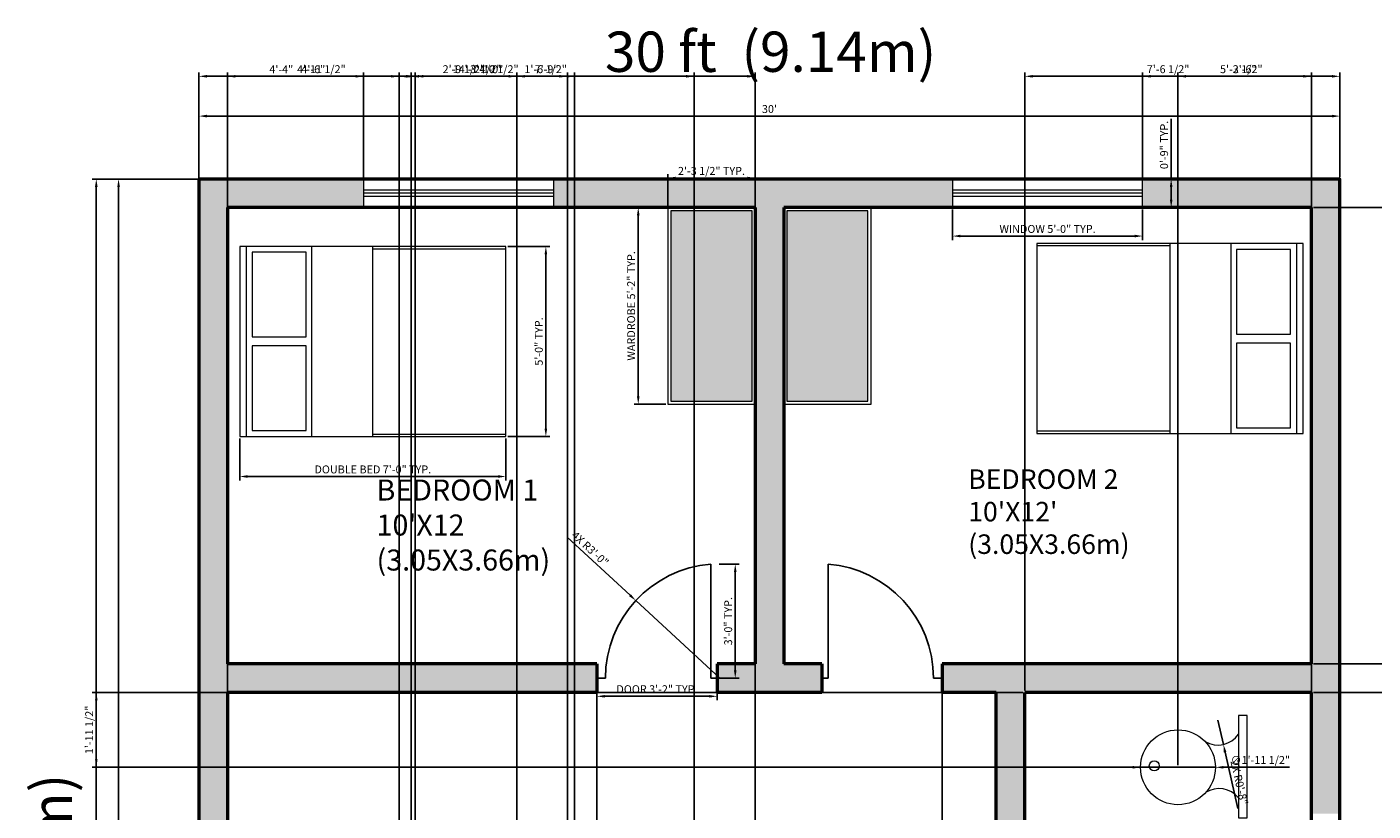
# Model space of a CAD drawing. Units: inches. Extents: x 655 to 1311, y 444 to 1096.
# Tile 3 of 4: x 655 to 1080, y 848 to 1096. Entities that reach past the tile are written whole.
import ezdxf

# ---------------------------------------------------------------- set-up
doc = ezdxf.new("R2010")
doc.units = ezdxf.units.IN
for name, color, linetype, lineweight in [('A-ANNO-DIMS', 7, 'Continuous', 18), ('A-AREA-IDEN', 7, 'Continuous', 18), ('A-COLS-PATT', 7, 'Continuous', 13), ('A-FLOR-FIXT', 8, 'Continuous', 18), ('A-WALL', 7, 'Continuous', 50), ('A-WALL-PATT', 7, 'Continuous', 13)]:
    doc.layers.add(name, color=color, linetype=linetype, lineweight=lineweight)
for name, color, linetype, lineweight, true_color in [('A-DOOR', 251, 'Continuous', 25, 0x636466), ('A-FURN', 251, 'Continuous', 18, 0x636466), ('A-FURN-PATT', 241, 'Continuous', 13, 0xf7abae), ('A-GLAZ', 152, 'Continuous', 18, 0x2776bb)]:
    doc.layers.add(name, color=color, linetype=linetype, lineweight=lineweight, true_color=true_color)
doc.styles.get("Standard").update_dxf_attribs({"font": 'arial.ttf'})
doc.dimstyles.new('ISO-25', dxfattribs={"dimtxt": 2.5, "dimasz": 2.5, "dimexe": 1.25, "dimexo": 0.625, "dimtad": 1, "dimdec": 0, "dimlunit": 3, "dimtxsty": 'Standard', "dimcen": 2.5, "dimadec": 0, "dimazin": 0, "dimtfac": 1, "dimtdec": 0, "dimtmove": 0, "dimatfit": 3, "dimfxl": 1, "dimarcsym": 0})

# ---------------------------------------------------------------- blocks, each defined once
blk = doc.blocks.new('*D1')
at = {"layer": 'A-ANNO-DIMS', "color": 0, "lineweight": -2, "transparency": 16777216}
for p, q in [((709.33, 1048.38), (709.33, 1068.85)), ((711.83, 1067.6), (1066.83, 1067.6)), ((1069.33, 1048.38), (1069.33, 1068.85))]:
    blk.add_line(p, q, dxfattribs=at)
at = {"layer": 'A-ANNO-DIMS', "color": 0, "transparency": 16777216}
for points in [[(711.83, 1068.02), (711.83, 1067.18), (709.33, 1067.6)], [(1066.83, 1068.02), (1066.83, 1067.18), (1069.33, 1067.6)]]:
    blk.add_solid(points, dxfattribs=at)
at = {"layer": 'Defpoints', "color": 0, "transparency": 16777216}
for p in [(1069.33, 1067.6), (709.33, 1047.75), (1069.33, 1047.75)]:
    blk.add_point(p, dxfattribs=at)
at = {"layer": 'A-ANNO-DIMS', "color": 0, "transparency": 16777216, "insert": (889.33, 1069.5), "char_height": 2.5, "attachment_point": 5}
blk.add_mtext("30'", dxfattribs=at)
blk = doc.blocks.new('*D2')
at = {"layer": 'A-ANNO-DIMS', "color": 0, "lineweight": -2, "transparency": 16777216}
for p, q in [((708.71, 1047.75), (682.71, 1047.75)), ((683.96, 570.25), (683.96, 1045.25)), ((708.71, 567.75), (682.71, 567.75))]:
    blk.add_line(p, q, dxfattribs=at)
at = {"layer": 'A-ANNO-DIMS', "color": 0, "transparency": 16777216}
for points in [[(683.55, 1045.25), (684.38, 1045.25), (683.96, 1047.75)], [(683.55, 570.25), (684.38, 570.25), (683.96, 567.75)]]:
    blk.add_solid(points, dxfattribs=at)
at = {"layer": 'Defpoints', "color": 0, "transparency": 16777216}
for p in [(683.96, 1047.75), (709.33, 1047.75), (709.33, 567.75)]:
    blk.add_point(p, dxfattribs=at)
at = {"layer": 'A-ANNO-DIMS', "color": 0, "transparency": 16777216, "insert": (682.06, 807.75), "char_height": 2.5, "attachment_point": 5, "rotation": 90}
blk.add_mtext("40'", dxfattribs=at)
blk = doc.blocks.new('DOOR-SWING-36IN')
for p, q in [((0, 0), (0, 36)), ((-36, 0), (-33.26, 0)), ((0, 0), (2, 0))]:
    blk.add_line(p, q)
blk.add_arc((2.86, 0), 36.11, 94.5377, 180)
blk = doc.blocks.new('WIN-60IN')
for p, q in [((60, 9), (0, 9)), ((0, 9), (0, 0)), ((60, 0), (60, 9)), ((60, 5.5), (0, 5.5)), ((60, 4.5), (0, 4.5)), ((60, 3.5), (0, 3.5)), ((0, 0), (60, 0))]:
    blk.add_line(p, q)
blk = doc.blocks.new('BED-DOUBLE')
for p, q in [((84, 60), (0, 60)), ((0, 60), (0, 0)), ((2, 60), (2, 0)), ((84, 0), (84, 60)), ((42, 59.26), (84, 59.26)), ((0, 0), (84, 0)), ((42, 0.79), (84, 0.79))]:
    blk.add_line(p, q)
for points in [[(42, 0), (42, 60), (22.65, 60), (22.65, 0)], [(20.99, 31.44), (20.99, 58.17), (3.97, 58.17), (3.97, 31.44)], [(20.99, 1.93), (20.99, 28.66), (3.97, 28.66), (3.97, 1.93)]]:
    blk.add_lwpolyline(points, close=True)
blk = doc.blocks.new('WARDROBE-BEDROOM')
for points in [[(27.59, 62.05), (0, 62.05), (0, 0), (27.59, 0)], [(26.59, 61.05), (1, 61.05), (1, 1), (26.59, 1)]]:
    blk.add_lwpolyline(points, close=True)
blk = doc.blocks.new('*D8')
at = {"layer": 'A-ANNO-DIMS', "color": 0, "lineweight": -2, "transparency": 16777216}
for p, q in [((834.83, 889.63), (834.83, 883.3)), ((872.83, 889.63), (872.83, 883.3)), ((837.33, 884.55), (870.33, 884.55))]:
    blk.add_line(p, q, dxfattribs=at)
at = {"layer": 'A-ANNO-DIMS', "color": 0, "transparency": 16777216}
for points in [[(837.33, 884.97), (837.33, 884.14), (834.83, 884.55)], [(870.33, 884.97), (870.33, 884.14), (872.83, 884.55)]]:
    blk.add_solid(points, dxfattribs=at)
at = {"layer": 'Defpoints', "color": 0, "transparency": 16777216}
for p in [(834.83, 890.25), (872.83, 890.25), (872.83, 884.55)]:
    blk.add_point(p, dxfattribs=at)
at = {"layer": 'A-ANNO-DIMS', "color": 0, "transparency": 16777216, "insert": (853.83, 886.47), "char_height": 2.5, "attachment_point": 5}
blk.add_mtext('DOOR 3\'-2" TYP.', dxfattribs=at)
blk = doc.blocks.new('*D9')
at = {"layer": 'A-ANNO-DIMS', "color": 0, "lineweight": -2, "transparency": 16777216}
for p, q in [((873.46, 926.25), (879.78, 926.25)), ((878.53, 892.75), (878.53, 923.75)), ((873.46, 890.25), (879.78, 890.25))]:
    blk.add_line(p, q, dxfattribs=at)
at = {"layer": 'A-ANNO-DIMS', "color": 0, "transparency": 16777216}
for points in [[(878.12, 923.75), (878.95, 923.75), (878.53, 926.25)], [(878.12, 892.75), (878.95, 892.75), (878.53, 890.25)]]:
    blk.add_solid(points, dxfattribs=at)
at = {"layer": 'Defpoints', "color": 0, "transparency": 16777216}
for p in [(872.83, 926.25), (878.53, 926.25), (872.83, 890.25)]:
    blk.add_point(p, dxfattribs=at)
at = {"layer": 'A-ANNO-DIMS', "color": 0, "transparency": 16777216, "insert": (876.63, 908.25), "char_height": 2.5, "attachment_point": 5, "rotation": 90}
blk.add_mtext('3\'-0" TYP.', dxfattribs=at)
blk = doc.blocks.new('*D10')
at = {"layer": 'A-ANNO-DIMS', "color": 0, "lineweight": -2, "transparency": 16777216}
for p, q in [((947.08, 1038.13), (947.08, 1028.5)), ((1007.08, 1038.13), (1007.08, 1028.5)), ((949.58, 1029.75), (1004.58, 1029.75))]:
    blk.add_line(p, q, dxfattribs=at)
at = {"layer": 'A-ANNO-DIMS', "color": 0, "transparency": 16777216}
for points in [[(949.58, 1030.17), (949.58, 1029.34), (947.08, 1029.75)], [(1004.58, 1030.17), (1004.58, 1029.34), (1007.08, 1029.75)]]:
    blk.add_solid(points, dxfattribs=at)
at = {"layer": 'Defpoints', "color": 0, "transparency": 16777216}
for p in [(947.08, 1038.75), (1007.08, 1038.75), (1007.08, 1029.75)]:
    blk.add_point(p, dxfattribs=at)
at = {"layer": 'A-ANNO-DIMS', "color": 0, "transparency": 16777216, "insert": (977.08, 1031.67), "char_height": 2.5, "attachment_point": 5}
blk.add_mtext('WINDOW 5\'-0" TYP.', dxfattribs=at)
blk = doc.blocks.new('*D11')
at = {"layer": 'A-ANNO-DIMS', "color": 0, "lineweight": -2, "transparency": 16777216}
for p, q in [((1016.08, 1047.75), (1016.08, 1066.74)), ((1007.71, 1047.75), (1017.33, 1047.75)), ((1016.08, 1041.25), (1016.08, 1045.25)), ((1007.71, 1038.75), (1017.33, 1038.75))]:
    blk.add_line(p, q, dxfattribs=at)
at = {"layer": 'A-ANNO-DIMS', "color": 0, "transparency": 16777216}
for points in [[(1015.67, 1045.25), (1016.5, 1045.25), (1016.08, 1047.75)], [(1015.67, 1041.25), (1016.5, 1041.25), (1016.08, 1038.75)]]:
    blk.add_solid(points, dxfattribs=at)
at = {"layer": 'Defpoints', "color": 0, "transparency": 16777216}
for p in [(1007.08, 1047.75), (1016.08, 1047.75), (1007.08, 1038.75)]:
    blk.add_point(p, dxfattribs=at)
at = {"layer": 'A-ANNO-DIMS', "color": 0, "transparency": 16777216, "insert": (1014.18, 1058.5), "char_height": 2.5, "attachment_point": 5, "rotation": 90}
blk.add_mtext('0\'-9" TYP.', dxfattribs=at)
blk = doc.blocks.new('*D12')
at = {"layer": 'A-ANNO-DIMS', "color": 0, "lineweight": -2, "transparency": 16777216}
for p, q in [((722.18, 965.87), (722.18, 952.64)), ((806.18, 965.87), (806.18, 952.64)), ((724.68, 953.89), (803.68, 953.89))]:
    blk.add_line(p, q, dxfattribs=at)
at = {"layer": 'A-ANNO-DIMS', "color": 0, "transparency": 16777216}
for points in [[(724.68, 954.31), (724.68, 953.48), (722.18, 953.89)], [(803.68, 954.31), (803.68, 953.48), (806.18, 953.89)]]:
    blk.add_solid(points, dxfattribs=at)
at = {"layer": 'Defpoints', "color": 0, "transparency": 16777216}
for p in [(722.18, 966.49), (806.18, 966.49), (806.18, 953.89)]:
    blk.add_point(p, dxfattribs=at)
at = {"layer": 'A-ANNO-DIMS', "color": 0, "transparency": 16777216, "insert": (764.18, 955.81), "char_height": 2.5, "attachment_point": 5}
blk.add_mtext('DOUBLE BED 7\'-0" TYP.', dxfattribs=at)
blk = doc.blocks.new('*D13')
at = {"layer": 'A-ANNO-DIMS', "color": 0, "lineweight": -2, "transparency": 16777216}
for p, q in [((806.8, 1026.49), (820.03, 1026.49)), ((818.78, 968.99), (818.78, 1023.99)), ((806.8, 966.49), (820.03, 966.49))]:
    blk.add_line(p, q, dxfattribs=at)
at = {"layer": 'A-ANNO-DIMS', "color": 0, "transparency": 16777216}
for points in [[(818.36, 1023.99), (819.19, 1023.99), (818.78, 1026.49)], [(818.36, 968.99), (819.19, 968.99), (818.78, 966.49)]]:
    blk.add_solid(points, dxfattribs=at)
at = {"layer": 'Defpoints', "color": 0, "transparency": 16777216}
for p in [(806.18, 1026.49), (818.78, 1026.49), (806.18, 966.49)]:
    blk.add_point(p, dxfattribs=at)
at = {"layer": 'A-ANNO-DIMS', "color": 0, "transparency": 16777216, "insert": (816.88, 996.49), "char_height": 2.5, "attachment_point": 5, "rotation": 90}
blk.add_mtext('5\'-0" TYP.', dxfattribs=at)
blk = doc.blocks.new('*D14')
at = {"layer": 'A-ANNO-DIMS', "color": 0, "lineweight": -2, "transparency": 16777216}
for p, q in [((856.62, 1038.75), (846.68, 1038.75)), ((847.93, 979.2), (847.93, 1036.25)), ((856.62, 976.7), (846.68, 976.7))]:
    blk.add_line(p, q, dxfattribs=at)
at = {"layer": 'A-ANNO-DIMS', "color": 0, "transparency": 16777216}
for points in [[(847.52, 1036.25), (848.35, 1036.25), (847.93, 1038.75)], [(847.52, 979.2), (848.35, 979.2), (847.93, 976.7)]]:
    blk.add_solid(points, dxfattribs=at)
at = {"layer": 'Defpoints', "color": 0, "transparency": 16777216}
for p in [(847.93, 1038.75), (857.24, 1038.75), (857.24, 976.7)]:
    blk.add_point(p, dxfattribs=at)
at = {"layer": 'A-ANNO-DIMS', "color": 0, "transparency": 16777216, "insert": (846.01, 1007.73), "char_height": 2.5, "attachment_point": 5, "rotation": 90}
blk.add_mtext('WARDROBE 5\'-2" TYP.', dxfattribs=at)
blk = doc.blocks.new('*D15')
at = {"layer": 'A-ANNO-DIMS', "color": 0, "lineweight": -2, "transparency": 16777216}
for p, q in [((857.24, 1039.38), (857.24, 1049.31)), ((884.83, 1039.38), (884.83, 1049.31)), ((859.74, 1048.06), (882.33, 1048.06))]:
    blk.add_line(p, q, dxfattribs=at)
at = {"layer": 'A-ANNO-DIMS', "color": 0, "transparency": 16777216}
for points in [[(859.74, 1048.48), (859.74, 1047.64), (857.24, 1048.06)], [(882.33, 1048.48), (882.33, 1047.64), (884.83, 1048.06)]]:
    blk.add_solid(points, dxfattribs=at)
at = {"layer": 'Defpoints', "color": 0, "transparency": 16777216}
for p in [(884.83, 1048.06), (857.24, 1038.75), (884.83, 1038.75)]:
    blk.add_point(p, dxfattribs=at)
at = {"layer": 'A-ANNO-DIMS', "color": 0, "transparency": 16777216, "insert": (871.04, 1049.98), "char_height": 2.5, "attachment_point": 5}
blk.add_mtext('2\'-3 1/2" TYP.', dxfattribs=at)
blk = doc.blocks.new('*D18')
at = {"layer": 'A-ANNO-DIMS', "color": 0, "lineweight": -2, "transparency": 16777216}
for p, q in [((718.33, 1039.38), (718.33, 1081.4)), ((720.83, 1080.15), (882.33, 1080.15)), ((884.83, 1039.38), (884.83, 1081.4))]:
    blk.add_line(p, q, dxfattribs=at)
at = {"layer": 'A-ANNO-DIMS', "color": 0, "transparency": 16777216}
for points in [[(720.83, 1080.57), (720.83, 1079.74), (718.33, 1080.15)], [(882.33, 1080.57), (882.33, 1079.74), (884.83, 1080.15)]]:
    blk.add_solid(points, dxfattribs=at)
at = {"layer": 'Defpoints', "color": 0, "transparency": 16777216}
for p in [(884.83, 1080.15), (718.33, 1038.75), (884.83, 1038.75)]:
    blk.add_point(p, dxfattribs=at)
at = {"layer": 'A-ANNO-DIMS', "color": 0, "transparency": 16777216, "insert": (801.58, 1082.07), "char_height": 2.5, "attachment_point": 5}
blk.add_mtext('13\'-10 1/2"', dxfattribs=at)
blk = doc.blocks.new('*D19')
at = {"layer": 'A-ANNO-DIMS', "color": 0, "lineweight": -2, "transparency": 16777216}
for p, q in [((709.33, 1048.38), (709.33, 1081.4)), ((711.83, 1080.15), (758.77, 1080.15)), ((761.27, 1048.38), (761.27, 1081.4))]:
    blk.add_line(p, q, dxfattribs=at)
at = {"layer": 'A-ANNO-DIMS', "color": 0, "transparency": 16777216}
for points in [[(711.83, 1080.57), (711.83, 1079.74), (709.33, 1080.15)], [(758.77, 1080.57), (758.77, 1079.74), (761.27, 1080.15)]]:
    blk.add_solid(points, dxfattribs=at)
at = {"layer": 'Defpoints', "color": 0, "transparency": 16777216}
for p in [(761.27, 1080.15), (709.33, 1047.75), (761.27, 1047.75)]:
    blk.add_point(p, dxfattribs=at)
at = {"layer": 'A-ANNO-DIMS', "color": 0, "transparency": 16777216, "insert": (735.3, 1082.03), "char_height": 2.5, "attachment_point": 5}
blk.add_mtext('4\'-4"', dxfattribs=at)
blk = doc.blocks.new('*D20')
at = {"layer": 'A-ANNO-DIMS', "color": 0, "lineweight": -2, "transparency": 16777216}
for p, q in [((1007.08, 1048.38), (1007.08, 1081.4)), ((1009.58, 1080.15), (1066.83, 1080.15)), ((1069.33, 1048.38), (1069.33, 1081.4))]:
    blk.add_line(p, q, dxfattribs=at)
at = {"layer": 'A-ANNO-DIMS', "color": 0, "transparency": 16777216}
for points in [[(1009.58, 1080.57), (1009.58, 1079.74), (1007.08, 1080.15)], [(1066.83, 1080.57), (1066.83, 1079.74), (1069.33, 1080.15)]]:
    blk.add_solid(points, dxfattribs=at)
at = {"layer": 'Defpoints', "color": 0, "transparency": 16777216}
for p in [(1069.33, 1080.15), (1007.08, 1047.75), (1069.33, 1047.75)]:
    blk.add_point(p, dxfattribs=at)
at = {"layer": 'A-ANNO-DIMS', "color": 0, "transparency": 16777216, "insert": (1038.21, 1082.07), "char_height": 2.5, "attachment_point": 5}
blk.add_mtext('5\'-2 1/2"', dxfattribs=at)
blk = doc.blocks.new('*D21')
at = {"layer": 'A-ANNO-DIMS', "color": 0, "lineweight": -2, "transparency": 16777216}
for p, q in [((718.33, 894.13), (718.33, 444.55)), ((834.83, 894.13), (834.83, 444.55)), ((720.83, 445.8), (832.33, 445.8))]:
    blk.add_line(p, q, dxfattribs=at)
at = {"layer": 'A-ANNO-DIMS', "color": 0, "transparency": 16777216}
for points in [[(720.83, 446.22), (720.83, 445.38), (718.33, 445.8)], [(832.33, 446.22), (832.33, 445.38), (834.83, 445.8)]]:
    blk.add_solid(points, dxfattribs=at)
at = {"layer": 'Defpoints', "color": 0, "transparency": 16777216}
for p in [(718.33, 894.75), (834.83, 894.75), (834.83, 445.8)]:
    blk.add_point(p, dxfattribs=at)
at = {"layer": 'A-ANNO-DIMS', "color": 0, "transparency": 16777216, "insert": (776.58, 447.72), "char_height": 2.5, "attachment_point": 5}
blk.add_mtext('9\'-8 1/2"', dxfattribs=at)
blk = doc.blocks.new('*D22')
at = {"layer": 'A-ANNO-DIMS', "color": 0, "lineweight": -2, "transparency": 16777216}
for p, q in [((943.83, 894.13), (943.83, 444.55)), ((1060.33, 894.13), (1060.33, 444.55)), ((946.33, 445.8), (1057.83, 445.8))]:
    blk.add_line(p, q, dxfattribs=at)
at = {"layer": 'A-ANNO-DIMS', "color": 0, "transparency": 16777216}
for points in [[(946.33, 446.22), (946.33, 445.38), (943.83, 445.8)], [(1057.83, 446.22), (1057.83, 445.38), (1060.33, 445.8)]]:
    blk.add_solid(points, dxfattribs=at)
at = {"layer": 'Defpoints', "color": 0, "transparency": 16777216}
for p in [(943.83, 894.75), (1060.33, 894.75), (1060.33, 445.8)]:
    blk.add_point(p, dxfattribs=at)
at = {"layer": 'A-ANNO-DIMS', "color": 0, "transparency": 16777216, "insert": (1002.08, 447.72), "char_height": 2.5, "attachment_point": 5}
blk.add_mtext('9\'-8 1/2"', dxfattribs=at)
blk = doc.blocks.new('*D23')
at = {"layer": 'A-ANNO-DIMS', "color": 0, "lineweight": -2, "transparency": 16777216}
for p, q in [((1060.96, 1038.75), (1102.98, 1038.75)), ((1101.73, 897.25), (1101.73, 1036.25)), ((1060.96, 894.75), (1102.98, 894.75))]:
    blk.add_line(p, q, dxfattribs=at)
at = {"layer": 'A-ANNO-DIMS', "color": 0, "transparency": 16777216}
for points in [[(1101.32, 1036.25), (1102.15, 1036.25), (1101.73, 1038.75)], [(1101.32, 897.25), (1102.15, 897.25), (1101.73, 894.75)]]:
    blk.add_solid(points, dxfattribs=at)
at = {"layer": 'Defpoints', "color": 0, "transparency": 16777216}
for p in [(1060.33, 1038.75), (1101.73, 1038.75), (1060.33, 894.75)]:
    blk.add_point(p, dxfattribs=at)
at = {"layer": 'A-ANNO-DIMS', "color": 0, "transparency": 16777216, "insert": (1099.83, 966.75), "char_height": 2.5, "attachment_point": 5, "rotation": 90}
blk.add_mtext('12\'-0"', dxfattribs=at)
blk = doc.blocks.new('*D24')
at = {"layer": 'A-ANNO-DIMS', "color": 0, "lineweight": -2, "transparency": 16777216}
for p, q in [((969.89, 886.38), (969.89, 1081.4)), ((972.39, 1080.15), (1057.83, 1080.15)), ((1060.33, 886.38), (1060.33, 1081.4))]:
    blk.add_line(p, q, dxfattribs=at)
at = {"layer": 'A-ANNO-DIMS', "color": 0, "transparency": 16777216}
for points in [[(972.39, 1080.57), (972.39, 1079.74), (969.89, 1080.15)], [(1057.83, 1080.57), (1057.83, 1079.74), (1060.33, 1080.15)]]:
    blk.add_solid(points, dxfattribs=at)
at = {"layer": 'Defpoints', "color": 0, "transparency": 16777216}
for p in [(1060.33, 1080.15), (969.89, 885.75), (1060.33, 885.75)]:
    blk.add_point(p, dxfattribs=at)
at = {"layer": 'A-ANNO-DIMS', "color": 0, "transparency": 16777216, "insert": (1015.11, 1082.07), "char_height": 2.5, "attachment_point": 5}
blk.add_mtext('7\'-6 1/2"', dxfattribs=at)
blk = doc.blocks.new('*D25')
at = {"layer": 'A-ANNO-DIMS', "color": 0, "lineweight": -2, "transparency": 16777216}
for p, q in [((1060.96, 885.75), (1102.98, 885.75)), ((1101.73, 765.73), (1101.73, 883.25)), ((1060.96, 763.23), (1102.98, 763.23))]:
    blk.add_line(p, q, dxfattribs=at)
at = {"layer": 'A-ANNO-DIMS', "color": 0, "transparency": 16777216}
for points in [[(1101.32, 883.25), (1102.15, 883.25), (1101.73, 885.75)], [(1101.32, 765.73), (1102.15, 765.73), (1101.73, 763.23)]]:
    blk.add_solid(points, dxfattribs=at)
at = {"layer": 'Defpoints', "color": 0, "transparency": 16777216}
for p in [(1060.33, 885.75), (1101.73, 885.75), (1060.33, 763.23)]:
    blk.add_point(p, dxfattribs=at)
at = {"layer": 'A-ANNO-DIMS', "color": 0, "transparency": 16777216, "insert": (1099.81, 824.49), "char_height": 2.5, "attachment_point": 5, "rotation": 90}
blk.add_mtext('10\'-2 1/2"', dxfattribs=at)
blk = doc.blocks.new('*D34')
at = {"layer": 'A-ANNO-DIMS', "color": 0, "lineweight": -2, "transparency": 16777216}
for p, q in [((1018.22, 862.78), (1018.22, 1081.4)), ((1020.72, 1080.15), (1057.83, 1080.15)), ((1060.33, 886.38), (1060.33, 1081.4))]:
    blk.add_line(p, q, dxfattribs=at)
at = {"layer": 'A-ANNO-DIMS', "color": 0, "transparency": 16777216}
for points in [[(1020.72, 1080.57), (1020.72, 1079.74), (1018.22, 1080.15)], [(1057.83, 1080.57), (1057.83, 1079.74), (1060.33, 1080.15)]]:
    blk.add_solid(points, dxfattribs=at)
at = {"layer": 'Defpoints', "color": 0, "transparency": 16777216}
for p in [(1060.33, 1080.15), (1060.33, 885.75), (1018.22, 862.16)]:
    blk.add_point(p, dxfattribs=at)
at = {"layer": 'A-ANNO-DIMS', "color": 0, "transparency": 16777216, "insert": (1039.27, 1082.06), "char_height": 2.5, "attachment_point": 5}
blk.add_mtext('3\'-6"', dxfattribs=at)
blk = doc.blocks.new('*D35')
at = {"layer": 'A-ANNO-DIMS', "color": 0, "lineweight": -2, "transparency": 16777216}
for p, q in [((969.27, 885.75), (675.68, 885.75)), ((676.93, 864.66), (676.93, 883.25)), ((1017.59, 862.16), (675.68, 862.16))]:
    blk.add_line(p, q, dxfattribs=at)
at = {"layer": 'A-ANNO-DIMS', "color": 0, "transparency": 16777216}
for points in [[(676.52, 883.25), (677.35, 883.25), (676.93, 885.75)], [(676.52, 864.66), (677.35, 864.66), (676.93, 862.16)]]:
    blk.add_solid(points, dxfattribs=at)
at = {"layer": 'Defpoints', "color": 0, "transparency": 16777216}
for p in [(676.93, 885.75), (969.89, 885.75), (1018.22, 862.16)]:
    blk.add_point(p, dxfattribs=at)
at = {"layer": 'A-ANNO-DIMS', "color": 0, "transparency": 16777216, "insert": (675.01, 873.96), "char_height": 2.5, "attachment_point": 5, "rotation": 90}
blk.add_mtext('1\'-11 1/2"', dxfattribs=at)
blk = doc.blocks.new('*D48')
at = {"layer": 'A-ANNO-DIMS', "color": 0, "lineweight": -2, "transparency": 16777216}
for p, q in [((709.33, 568.38), (709.33, 1081.4)), ((711.83, 1080.15), (882.33, 1080.15)), ((884.83, 568.38), (884.83, 1081.4))]:
    blk.add_line(p, q, dxfattribs=at)
at = {"layer": 'A-ANNO-DIMS', "color": 0, "transparency": 16777216}
for points in [[(711.83, 1080.57), (711.83, 1079.74), (709.33, 1080.15)], [(882.33, 1080.57), (882.33, 1079.74), (884.83, 1080.15)]]:
    blk.add_solid(points, dxfattribs=at)
at = {"layer": 'Defpoints', "color": 0, "transparency": 16777216}
for p in [(884.83, 1080.15), (709.33, 567.75), (884.83, 567.75)]:
    blk.add_point(p, dxfattribs=at)
at = {"layer": 'A-ANNO-DIMS', "color": 0, "transparency": 16777216, "insert": (797.08, 1082.07), "char_height": 2.5, "attachment_point": 5}
blk.add_mtext('14\'-7 1/2"', dxfattribs=at)
blk = doc.blocks.new('*D51')
at = {"layer": 'A-ANNO-DIMS', "color": 0, "lineweight": -2, "transparency": 16777216}
for p, q in [((718.33, 559.38), (718.33, 1081.4)), ((720.83, 1080.15), (775.08, 1080.15)), ((777.58, 559.38), (777.58, 1081.4))]:
    blk.add_line(p, q, dxfattribs=at)
at = {"layer": 'A-ANNO-DIMS', "color": 0, "transparency": 16777216}
for points in [[(720.83, 1080.57), (720.83, 1079.74), (718.33, 1080.15)], [(775.08, 1080.57), (775.08, 1079.74), (777.58, 1080.15)]]:
    blk.add_solid(points, dxfattribs=at)
at = {"layer": 'Defpoints', "color": 0, "transparency": 16777216}
for p in [(777.58, 1080.15), (718.33, 558.75), (777.58, 558.75)]:
    blk.add_point(p, dxfattribs=at)
at = {"layer": 'A-ANNO-DIMS', "color": 0, "transparency": 16777216, "insert": (747.96, 1082.07), "char_height": 2.5, "attachment_point": 5}
blk.add_mtext('4\'-11 1/2"', dxfattribs=at)
blk = doc.blocks.new('*D53')
at = {"layer": 'A-ANNO-DIMS', "color": 0, "lineweight": -2, "transparency": 16777216}
for p, q in [((777.58, 527.53), (777.58, 1081.4)), ((780.08, 1080.15), (823.08, 1080.15)), ((825.58, 527.53), (825.58, 1081.4))]:
    blk.add_line(p, q, dxfattribs=at)
at = {"layer": 'A-ANNO-DIMS', "color": 0, "transparency": 16777216}
for points in [[(780.08, 1080.57), (780.08, 1079.74), (777.58, 1080.15)], [(823.08, 1080.57), (823.08, 1079.74), (825.58, 1080.15)]]:
    blk.add_solid(points, dxfattribs=at)
at = {"layer": 'Defpoints', "color": 0, "transparency": 16777216}
for p in [(825.58, 1080.15), (777.58, 526.9), (825.58, 526.9)]:
    blk.add_point(p, dxfattribs=at)
at = {"layer": 'A-ANNO-DIMS', "color": 0, "transparency": 16777216, "insert": (801.58, 1082.05), "char_height": 2.5, "attachment_point": 5}
blk.add_mtext('4\'-0"', dxfattribs=at)
blk = doc.blocks.new('*D54')
at = {"layer": 'A-ANNO-DIMS', "color": 0, "lineweight": -2, "transparency": 16777216}
for p, q in [((708.71, 1047.75), (675.68, 1047.75)), ((676.93, 480.7), (676.93, 1045.25)), ((708.71, 478.2), (675.68, 478.2))]:
    blk.add_line(p, q, dxfattribs=at)
at = {"layer": 'A-ANNO-DIMS', "color": 0, "transparency": 16777216}
for points in [[(676.52, 1045.25), (677.35, 1045.25), (676.93, 1047.75)], [(676.52, 480.7), (677.35, 480.7), (676.93, 478.2)]]:
    blk.add_solid(points, dxfattribs=at)
at = {"layer": 'Defpoints', "color": 0, "transparency": 16777216}
for p in [(676.93, 1047.75), (709.33, 1047.75), (709.33, 478.2)]:
    blk.add_point(p, dxfattribs=at)
at = {"layer": 'A-ANNO-DIMS', "color": 0, "transparency": 16777216, "insert": (675.01, 762.98), "char_height": 2.5, "attachment_point": 5, "rotation": 90}
blk.add_mtext('47\'-5 1/2"', dxfattribs=at)
blk = doc.blocks.new('*D55')
at = {"layer": 'A-ANNO-DIMS', "color": 0, "lineweight": -2, "transparency": 16777216}
for p, q in [((772.49, 690.25), (772.49, 1081.4)), ((774.99, 1080.15), (863.04, 1080.15)), ((865.54, 690.25), (865.54, 1081.4))]:
    blk.add_line(p, q, dxfattribs=at)
at = {"layer": 'A-ANNO-DIMS', "color": 0, "transparency": 16777216}
for points in [[(774.99, 1080.57), (774.99, 1079.74), (772.49, 1080.15)], [(863.04, 1080.57), (863.04, 1079.74), (865.54, 1080.15)]]:
    blk.add_solid(points, dxfattribs=at)
at = {"layer": 'Defpoints', "color": 0, "transparency": 16777216}
for p in [(865.54, 1080.15), (772.49, 689.62), (865.54, 689.62)]:
    blk.add_point(p, dxfattribs=at)
at = {"layer": 'A-ANNO-DIMS', "color": 0, "transparency": 16777216, "insert": (819.01, 1082.05), "char_height": 2.5, "attachment_point": 5}
blk.add_mtext('7\'-9"', dxfattribs=at)
blk = doc.blocks.new('*D57')
at = {"layer": 'A-ANNO-DIMS', "color": 0, "lineweight": -2, "transparency": 16777216}
for p, q in [((776.25, 816.16), (776.25, 1081.4)), ((778.75, 1080.15), (807.08, 1080.15)), ((809.58, 816.16), (809.58, 1081.4))]:
    blk.add_line(p, q, dxfattribs=at)
at = {"layer": 'A-ANNO-DIMS', "color": 0, "transparency": 16777216}
for points in [[(778.75, 1080.57), (778.75, 1079.74), (776.25, 1080.15)], [(807.08, 1080.57), (807.08, 1079.74), (809.58, 1080.15)]]:
    blk.add_solid(points, dxfattribs=at)
at = {"layer": 'Defpoints', "color": 0, "transparency": 16777216}
for p in [(809.58, 1080.15), (776.25, 815.54), (809.58, 815.54)]:
    blk.add_point(p, dxfattribs=at)
at = {"layer": 'A-ANNO-DIMS', "color": 0, "transparency": 16777216, "insert": (792.91, 1082.07), "char_height": 2.5, "attachment_point": 5}
blk.add_mtext('2\'-9 1/2"', dxfattribs=at)
blk = doc.blocks.new('*D59')
at = {"layer": 'A-ANNO-DIMS', "color": 0, "lineweight": -2, "transparency": 16777216}
for p, q in [((718.33, 658.38), (718.33, 1081.4)), ((720.83, 1080.15), (769.99, 1080.15)), ((772.49, 690.25), (772.49, 1081.4))]:
    blk.add_line(p, q, dxfattribs=at)
at = {"layer": 'A-ANNO-DIMS', "color": 0, "transparency": 16777216}
for points in [[(720.83, 1080.57), (720.83, 1079.74), (718.33, 1080.15)], [(769.99, 1080.57), (769.99, 1079.74), (772.49, 1080.15)]]:
    blk.add_solid(points, dxfattribs=at)
at = {"layer": 'Defpoints', "color": 0, "transparency": 16777216}
for p in [(772.49, 1080.15), (772.49, 689.62), (718.33, 657.75)]:
    blk.add_point(p, dxfattribs=at)
at = {"layer": 'A-ANNO-DIMS', "color": 0, "transparency": 16777216, "insert": (745.41, 1082.05), "char_height": 2.5, "attachment_point": 5}
blk.add_mtext('4\'-6"', dxfattribs=at)
blk = doc.blocks.new('*D61')
at = {"layer": 'A-ANNO-DIMS', "color": 0, "lineweight": -2, "transparency": 16777216}
for p, q in [((809.58, 816.16), (809.58, 1081.4)), ((812.08, 1080.15), (825.34, 1080.15)), ((827.84, 831.58), (827.84, 1081.4))]:
    blk.add_line(p, q, dxfattribs=at)
at = {"layer": 'A-ANNO-DIMS', "color": 0, "transparency": 16777216}
for points in [[(812.08, 1080.57), (812.08, 1079.74), (809.58, 1080.15)], [(825.34, 1080.57), (825.34, 1079.74), (827.84, 1080.15)]]:
    blk.add_solid(points, dxfattribs=at)
at = {"layer": 'Defpoints', "color": 0, "transparency": 16777216}
for p in [(827.84, 1080.15), (827.84, 830.95), (809.58, 815.54)]:
    blk.add_point(p, dxfattribs=at)
at = {"layer": 'A-ANNO-DIMS', "color": 0, "transparency": 16777216, "insert": (818.71, 1082.07), "char_height": 2.5, "attachment_point": 5}
blk.add_mtext('1\'-6 1/2"', dxfattribs=at)
blk = doc.blocks.new('*D63')
at = {"layer": 'A-ANNO-DIMS', "color": 0, "lineweight": -2, "transparency": 16777216}
for p, q in [((825.46, 934.81), (845.33, 916.45)), ((873.69, 890.25), (847.16, 914.76))]:
    blk.add_line(p, q, dxfattribs=at)
at = {"layer": 'A-ANNO-DIMS', "color": 0, "transparency": 16777216}
blk.add_solid([(845.61, 916.76), (845.04, 916.15), (847.16, 914.76)], dxfattribs=at)
at = {"layer": 'Defpoints', "color": 0, "transparency": 16777216}
for p in [(847.16, 914.76), (873.69, 890.25)]:
    blk.add_point(p, dxfattribs=at)
at = {"layer": 'A-ANNO-DIMS', "color": 0, "transparency": 16777216, "insert": (832.54, 930.86), "char_height": 2.5, "attachment_point": 5, "rotation": 317.2687}
blk.add_mtext('4X R3\'-0"', dxfattribs=at)
blk = doc.blocks.new('*D65')
at = {"layer": 'A-ANNO-DIMS', "color": 0, "lineweight": -2, "transparency": 16777216}
for p, q in [((1003.9, 862.16), (1001.4, 862.16)), ((1006.4, 862.16), (1030.04, 862.16)), ((1053.42, 862.16), (1032.54, 862.16))]:
    blk.add_line(p, q, dxfattribs=at)
at = {"layer": 'A-ANNO-DIMS', "color": 0, "transparency": 16777216}
for points in [[(1003.9, 862.58), (1003.9, 861.74), (1006.4, 862.16)], [(1032.54, 862.57), (1032.54, 861.74), (1030.04, 862.16)]]:
    blk.add_solid(points, dxfattribs=at)
at = {"layer": 'Defpoints', "color": 0, "transparency": 16777216}
for p in [(1006.4, 862.16), (1030.04, 862.16)]:
    blk.add_point(p, dxfattribs=at)
at = {"layer": 'A-ANNO-DIMS', "color": 0, "transparency": 16777216, "insert": (1044.23, 864.13), "char_height": 2.5, "attachment_point": 5, "rotation": 359.9987}
blk.add_mtext('∅1\'-11 1/2"', dxfattribs=at)
blk = doc.blocks.new('*D66')
at = {"layer": 'A-ANNO-DIMS', "color": 0, "lineweight": -2, "transparency": 16777216}
for p, q in [((1030.8, 877.06), (1032.55, 869.37)), ((1037.16, 849.19), (1033.11, 866.93))]:
    blk.add_line(p, q, dxfattribs=at)
at = {"layer": 'A-ANNO-DIMS', "color": 0, "transparency": 16777216}
blk.add_solid([(1033.52, 867.03), (1032.7, 866.84), (1032.55, 869.37)], dxfattribs=at)
at = {"layer": 'Defpoints', "color": 0, "transparency": 16777216}
for p in [(1030.8, 877.06), (1032.55, 869.37)]:
    blk.add_point(p, dxfattribs=at)
at = {"layer": 'A-ANNO-DIMS', "color": 0, "transparency": 16777216, "insert": (1037.26, 857.26), "char_height": 2.5, "attachment_point": 5, "rotation": 282.8435}
blk.add_mtext('2X R0\'-8"', dxfattribs=at)

msp = doc.modelspace()

# ---------------------------------------------------------------- hatches: boundary and pattern name
at = {"layer": 'A-COLS-PATT'}
h = msp.add_hatch(color=256, dxfattribs=at)
h.dxf.hatch_style = 1
h.paths.add_polyline_path([(718.33, 558.75), (718.33, 567.75), (709.33, 567.75), (709.33, 558.75)])
h.paths.add_polyline_path([(893.83, 567.75), (884.83, 567.75), (884.83, 558.75), (893.83, 558.75)])
h.paths.add_polyline_path([(875.1, 756.19), (944.53, 756.19), (944.53, 796.18), (875.1, 796.18)], flags=9)
h.paths.add_polyline_path([(997.04, 810.04), (1045.86, 810.04), (1045.86, 839.51), (997.04, 839.51)], flags=9)
h.paths.add_polyline_path([(949.57, 925.87), (1005.17, 925.87), (1005.17, 959.21), (949.57, 959.21)], flags=9)
h.paths.add_polyline_path([(762.7, 920.37), (822.54, 920.37), (822.54, 956.25), (762.7, 956.25)], flags=9)
at = {"layer": 'A-FURN-PATT'}
h = msp.add_hatch(color=256, dxfattribs=at)
h.dxf.hatch_style = 1
h.paths.add_polyline_path([(883.83, 1037.75), (858.24, 1037.75), (858.24, 977.7), (883.83, 977.7)])
h.paths.add_polyline_path([(920.42, 1037.75), (894.83, 1037.75), (894.83, 977.7), (920.42, 977.7)])
at = {"layer": 'A-WALL-PATT'}
h = msp.add_hatch(color=256, dxfattribs=at)
h.dxf.hatch_style = 1
h.paths.add_polyline_path([(969.89, 885.75), (1060.33, 885.75), (1060.33, 847.5), (1069.33, 847.5), (1069.33, 1047.75), (1007.08, 1047.75), (1007.08, 1038.75), (1060.33, 1038.75), (1060.33, 894.75), (943.83, 894.75), (943.83, 885.75), (960.89, 885.75), (960.89, 822.23), (969.89, 822.23)])
h.paths.add_polyline_path([(969.89, 780.75), (969.89, 790.23), (960.89, 790.23), (960.89, 733.85), (893.83, 733.85), (893.83, 695.8), (902.83, 695.71), (902.83, 724.85), (969.89, 724.85), (969.89, 754.19), (1060.33, 754.19), (1060.33, 699.99), (1069.33, 699.99), (1069.33, 823.5), (1060.33, 823.5), (1060.33, 763.19), (969.89, 763.19)])
h.paths.add_polyline_path([(947.08, 1047.75), (821.27, 1047.75), (821.27, 1038.75), (884.83, 1038.75), (884.83, 976.7), (884.83, 894.75), (872.83, 894.75), (872.83, 885.75), (905.83, 885.75), (905.83, 894.75), (893.83, 894.75), (893.83, 1038.75), (921.42, 1038.75), (947.08, 1038.75)])
h.paths.add_polyline_path([(761.27, 1047.75), (709.33, 1047.75), (709.33, 648.75), (736.08, 648.75), (736.08, 657.75), (718.33, 657.75), (718.33, 885.75), (834.83, 885.75), (834.83, 894.75), (718.33, 894.75), (718.33, 1038.75), (761.27, 1038.75)])
h.paths.add_polyline_path([(822.83, 657.75), (796.08, 657.75), (796.08, 648.75), (822.83, 648.75)], flags=17)
h.paths.add_polyline_path([(893.83, 657.75), (860.83, 657.75), (860.83, 648.75), (884.83, 648.75), (884.83, 567.75), (893.83, 567.75)])
h.paths.add_polyline_path([(902.83, 657.75), (893.83, 657.75), (893.83, 567.75), (1069.33, 567.75), (1069.33, 639.99), (1060.33, 639.99), (1060.33, 576.75), (902.83, 576.75)])

# ---------------------------------------------------------------- linework, layer by layer
at = {"layer": 'A-FLOR-FIXT'}
msp.add_lwpolyline([(1037.33, 846.23), (1040.06, 846.23), (1040.06, 878.53), (1037.33, 878.53)], close=True, dxfattribs=at)
for centre, radius in [((1018.22, 862.16), 11.82), ((1010.75, 862.61), 1.58)]:
    msp.add_circle(centre, radius, dxfattribs=at)
for centre, start, end in [((1030.8, 877.06), 239.8163, 325.8719), ((1031.21, 847.55), 39.0557, 122.8464)]:
    msp.add_arc(centre, 7.88, start, end, dxfattribs=at)
at = {"layer": 'A-WALL'}
for p, q in [((718.33, 1038.75), (718.33, 894.75)), ((884.83, 1038.75), (718.33, 1038.75)), ((884.83, 1038.75), (884.83, 894.75)), ((1060.33, 1038.75), (893.83, 1038.75)), ((893.83, 1038.75), (893.83, 894.75)), ((1060.33, 894.75), (1060.33, 1038.75)), ((834.83, 894.75), (718.33, 894.75)), ((834.83, 894.75), (834.83, 885.75)), ((884.83, 894.75), (872.83, 894.75)), ((872.83, 894.75), (872.83, 885.75)), ((905.83, 894.75), (893.83, 894.75)), ((905.83, 894.75), (905.83, 885.75)), ((1060.33, 894.75), (943.83, 894.75)), ((943.83, 894.75), (943.83, 885.75)), ((834.83, 885.75), (718.33, 885.75)), ((718.33, 885.75), (718.33, 657.75)), ((905.83, 885.75), (872.83, 885.75)), ((960.89, 885.75), (943.83, 885.75)), ((960.89, 822.23), (960.89, 885.75)), ((1060.33, 885.75), (969.89, 885.75)), ((969.89, 822.23), (969.89, 885.75)), ((1060.33, 763.19), (1060.33, 885.75))]:
    msp.add_line(p, q, dxfattribs=at)
msp.add_lwpolyline([(893.83, 567.75), (1069.33, 567.75), (1069.33, 1047.75), (709.33, 1047.75), (709.33, 567.75)], dxfattribs=at)

# ---------------------------------------------------------------- block references
at = {"layer": 'A-DOOR'}
msp.add_blockref('DOOR-SWING-36IN', (870.83, 890.25), dxfattribs=at)
at = {"layer": 'A-DOOR', "extrusion": (0, 0, -1), "zscale": -1}
msp.add_blockref('DOOR-SWING-36IN', (-907.83, 890.25), dxfattribs=at)
at = {"layer": 'A-FURN'}
for name, p in [('WARDROBE-BEDROOM', (857.24, 976.7)), ('WARDROBE-BEDROOM', (893.83, 976.7)), ('BED-DOUBLE', (722.18, 966.49))]:
    msp.add_blockref(name, p, dxfattribs=at)
at = {"layer": 'A-FURN', "rotation": 180}
msp.add_blockref('BED-DOUBLE', (1057.7, 1027.42), dxfattribs=at)
at = {"layer": 'A-GLAZ'}
for p in [(761.27, 1038.75), (947.08, 1038.75)]:
    msp.add_blockref('WIN-60IN', p, dxfattribs=at)

# ---------------------------------------------------------------- texts
at = {"layer": 'A-ANNO-DIMS', "insert": (837.41, 1094.26), "char_height": 12.7117, "attachment_point": 1}
msp.add_mtext_dynamic_manual_height_columns('30 ft  (9.14m)', width=400.2868, gutter_width=63.56, heights=[0], dxfattribs=at)
at = {"layer": 'A-ANNO-DIMS', "insert": (656.52, 736.3), "char_height": 12.7117, "attachment_point": 1, "rotation": 90}
msp.add_mtext_dynamic_manual_height_columns('40 ft  (12.192m)', width=400.2868, gutter_width=63.56, heights=[0], dxfattribs=at)
at = {"layer": 'A-AREA-IDEN', "attachment_point": 1}
for s, width, gutter_width, insert, char_height in [("BEDROOM 2\\P10'X12'\\P(3.05X3.66m)", 219.6759, 30.78, (952.05, 956.15), 6.1564), ("BEDROOM 1\\P10'X12\\P(3.05X3.66m)", 228.5395, 33.13, (765.36, 952.95), 6.6256)]:
    msp.add_mtext_dynamic_manual_height_columns(s, width=width, gutter_width=gutter_width, heights=[0], dxfattribs=dict(at, insert=insert, char_height=char_height))

# ---------------------------------------------------------------- dimensions: what is measured, and where the dimension line sits
at = {"layer": 'A-ANNO-DIMS'}
for base, p1, p2, override, picture, middle in [((884.83, 1080.15), (709.33, 567.75), (884.83, 567.75), {"dimdec": 1, "dimlfac": 1, "dimrnd": 0, "dimzin": 1, "dimdsep": 46, "dimlunit": 4, "dimfrac": 2}, '*D48', (797.08, 1082.07)), ((761.27, 1080.15), (709.33, 1047.75), (761.27, 1047.75), {"dimdec": 1, "dimlfac": 1, "dimrnd": 0, "dimzin": 1, "dimdsep": 46, "dimlunit": 4, "dimfrac": 2}, '*D19', (735.3, 1082.03)), ((884.83, 1080.15), (718.33, 1038.75), (884.83, 1038.75), {"dimdec": 1, "dimlfac": 1, "dimrnd": 0, "dimzin": 1, "dimdsep": 46, "dimlunit": 4, "dimfrac": 2}, '*D18', (801.58, 1082.07)), ((777.582624, 1080.153006), (718.332624, 558.753006), (777.582624, 558.753006), {"dimdec": 1, "dimlfac": 1, "dimrnd": 0, "dimzin": 1, "dimdsep": 46, "dimlunit": 4, "dimfrac": 2}, '*D51', (747.957624, 1082.07063902)), ((772.49, 1080.15), (718.33, 657.75), (772.49, 689.62), {"dimdec": 1, "dimlfac": 1, "dimrnd": 0, "dimzin": 1, "dimdsep": 46, "dimlunit": 4, "dimfrac": 2}, '*D59', (745.41, 1082.05)), ((865.5433, 1080.153), (772.4866, 689.6218), (865.5433, 689.6218), {"dimdec": 1, "dimlfac": 1, "dimrnd": 0, "dimzin": 1, "dimdsep": 46, "dimlunit": 4, "dimfrac": 2}, '*D55', (819.0149, 1082.0544)), ((809.58, 1080.15), (776.25, 815.54), (809.58, 815.54), {"dimdec": 1, "dimlfac": 1, "dimrnd": 0, "dimzin": 1, "dimdsep": 46, "dimlunit": 4, "dimfrac": 2}, '*D57', (792.91, 1082.07)), ((825.58, 1080.15), (777.58, 526.9), (825.58, 526.9), {"dimdec": 1, "dimlfac": 1, "dimrnd": 0, "dimzin": 1, "dimdsep": 46, "dimlunit": 4, "dimfrac": 2}, '*D53', (801.58, 1082.05)), ((827.84, 1080.15), (809.58, 815.54), (827.84, 830.95), {"dimdec": 1, "dimlfac": 1, "dimrnd": 0, "dimzin": 1, "dimdsep": 46, "dimlunit": 4, "dimfrac": 2}, '*D61', (818.71, 1082.07)), ((1060.33, 1080.15), (969.89, 885.75), (1060.33, 885.75), {"dimdec": 1, "dimlfac": 1, "dimrnd": 0, "dimzin": 1, "dimdsep": 46, "dimlunit": 4, "dimfrac": 2}, '*D24', (1015.11, 1082.07)), ((1069.332624, 1080.153006), (1007.082624, 1047.753006), (1069.332624, 1047.753006), {"dimdec": 1, "dimlfac": 1, "dimrnd": 0, "dimzin": 1, "dimdsep": 46, "dimlunit": 4, "dimfrac": 2}, '*D20', (1038.207624, 1082.07063902)), ((1060.33, 1080.15), (1018.22, 862.16), (1060.33, 885.75), {"dimdec": 1, "dimlfac": 1, "dimrnd": 0, "dimzin": 1, "dimdsep": 46, "dimlunit": 4, "dimfrac": 2}, '*D34', (1039.27, 1082.06)), ((1069.33, 1067.6), (709.33, 1047.75), (1069.33, 1047.75), {"dimclrd": 0, "dimclre": 0, "dimclrt": 0}, '*D1', (889.33, 1069.5)), ((834.83, 445.8), (718.33, 894.75), (834.83, 894.75), {"dimdec": 1, "dimlfac": 1, "dimrnd": 0, "dimzin": 1, "dimdsep": 46, "dimlunit": 4, "dimfrac": 2}, '*D21', (776.58, 447.72)), ((1060.33, 445.8), (943.83, 894.75), (1060.33, 894.75), {"dimdec": 1, "dimlfac": 1, "dimrnd": 0, "dimzin": 1, "dimdsep": 46, "dimlunit": 4, "dimfrac": 2}, '*D22', (1002.08, 447.72))]:
    dim = msp.add_linear_dim(base=base, p1=p1, p2=p2, dimstyle='ISO-25', override=override, dxfattribs=at)
    dim.commit()
    dim.dimension.update_dxf_attribs({"geometry": picture, "text_midpoint": middle})
for base, p1, p2, text, picture, middle in [((1016.08, 1047.75), (1007.08, 1038.75), (1007.08, 1047.75), '<> TYP.', '*D11', (1014.18, 1058.5)), ((847.9332, 1038.753), (857.2412, 976.6996), (857.2412, 1038.753), 'WARDROBE <> TYP.', '*D14', (846.0147, 1007.7263)), ((818.78, 1026.49), (806.18, 966.49), (806.18, 1026.49), '<> TYP.', '*D13', (816.88, 996.49)), ((878.53, 926.25), (872.83, 890.25), (872.83, 926.25), '<> TYP.', '*D9', (876.63, 908.25))]:
    dim = msp.add_linear_dim(base=base, p1=p1, p2=p2, angle=90, text=text, dimstyle='ISO-25', override={"dimdec": 1, "dimlfac": 1, "dimrnd": 0, "dimzin": 1, "dimdsep": 46, "dimlunit": 4, "dimfrac": 2}, dxfattribs=at)
    dim.commit()
    dim.dimension.update_dxf_attribs({"geometry": picture, "text_midpoint": middle})
for base, p1, p2, text, picture, middle in [((884.83, 1048.06), (857.24, 1038.75), (884.83, 1038.75), '<> TYP.', '*D15', (871.04, 1049.98)), ((1007.08, 1029.75), (947.08, 1038.75), (1007.08, 1038.75), 'WINDOW <> TYP.', '*D10', (977.08, 1031.67)), ((806.18, 953.89), (722.18, 966.49), (806.18, 966.49), 'DOUBLE BED <> TYP.', '*D12', (764.18, 955.81)), ((872.83, 884.55), (834.83, 890.25), (872.83, 890.25), 'DOOR <> TYP.', '*D8', (853.83, 886.47))]:
    dim = msp.add_linear_dim(base=base, p1=p1, p2=p2, text=text, dimstyle='ISO-25', override={"dimdec": 1, "dimlfac": 1, "dimrnd": 0, "dimzin": 1, "dimdsep": 46, "dimlunit": 4, "dimfrac": 2}, dxfattribs=at)
    dim.commit()
    dim.dimension.update_dxf_attribs({"geometry": picture, "text_midpoint": middle})
for base, p1, p2, override, picture, middle in [((676.9326, 1047.753), (709.3326, 478.201), (709.3326, 1047.753), {"dimdec": 1, "dimlfac": 1, "dimrnd": 0, "dimzin": 1, "dimdsep": 46, "dimlunit": 4, "dimfrac": 2}, '*D54', (675.015, 762.977)), ((683.96, 1047.75), (709.33, 567.75), (709.33, 1047.75), {"dimclrd": 0, "dimclre": 0, "dimclrt": 0}, '*D2', (682.06, 807.75)), ((1101.73, 1038.75), (1060.33, 894.75), (1060.33, 1038.75), {"dimdec": 1, "dimlfac": 1, "dimrnd": 0, "dimzin": 1, "dimdsep": 46, "dimlunit": 4, "dimfrac": 2}, '*D23', (1099.83, 966.75)), ((676.93, 885.75), (1018.22, 862.16), (969.89, 885.75), {"dimdec": 1, "dimlfac": 1, "dimrnd": 0, "dimzin": 1, "dimdsep": 46, "dimlunit": 4, "dimfrac": 2}, '*D35', (675.01, 873.96)), ((1101.73, 885.75), (1060.33, 763.23), (1060.33, 885.75), {"dimdec": 1, "dimlfac": 1, "dimrnd": 0, "dimzin": 1, "dimdsep": 46, "dimlunit": 4, "dimfrac": 2}, '*D25', (1099.81, 824.49))]:
    dim = msp.add_linear_dim(base=base, p1=p1, p2=p2, angle=90, dimstyle='ISO-25', override=override, dxfattribs=at)
    dim.commit()
    dim.dimension.update_dxf_attribs({"geometry": picture, "text_midpoint": middle})
dim = msp.add_radius_dim(center=(873.69, 890.25), mpoint=(847.16, 914.76), text='4X <>', dimstyle='ISO-25', override={"dimdec": 1, "dimlfac": 1, "dimrnd": 0, "dimzin": 1, "dimdsep": 46, "dimlunit": 4, "dimfrac": 2}, dxfattribs=at)
dim.commit()
dim.dimension.update_dxf_attribs({"geometry": '*D63', "text_midpoint": (831.25, 929.46), "dimtype": 164})
dim = msp.add_radius_dim(center=(1030.8, 877.06), mpoint=(1032.55, 869.37), text='2X <>', dimstyle='ISO-25', override={"dimdec": 1, "dimlfac": 1, "dimrnd": 0, "dimzin": 1, "dimdsep": 46, "dimlunit": 4, "dimfrac": 2}, dxfattribs=at)
dim.commit()
dim.dimension.update_dxf_attribs({"geometry": '*D66', "text_midpoint": (1037.26, 857.26)})
dim = msp.add_diameter_dim_2p(p1=(1006.4, 862.16), p2=(1030.04, 862.16), dimstyle='ISO-25', override={"dimdec": 1, "dimlfac": 1, "dimrnd": 0, "dimzin": 1, "dimdsep": 46, "dimlunit": 4, "dimfrac": 2}, dxfattribs=at)
dim.commit()
dim.dimension.update_dxf_attribs({"geometry": '*D65', "text_midpoint": (1044.23, 862.16)})

doc.saveas('drawing.dxf')
